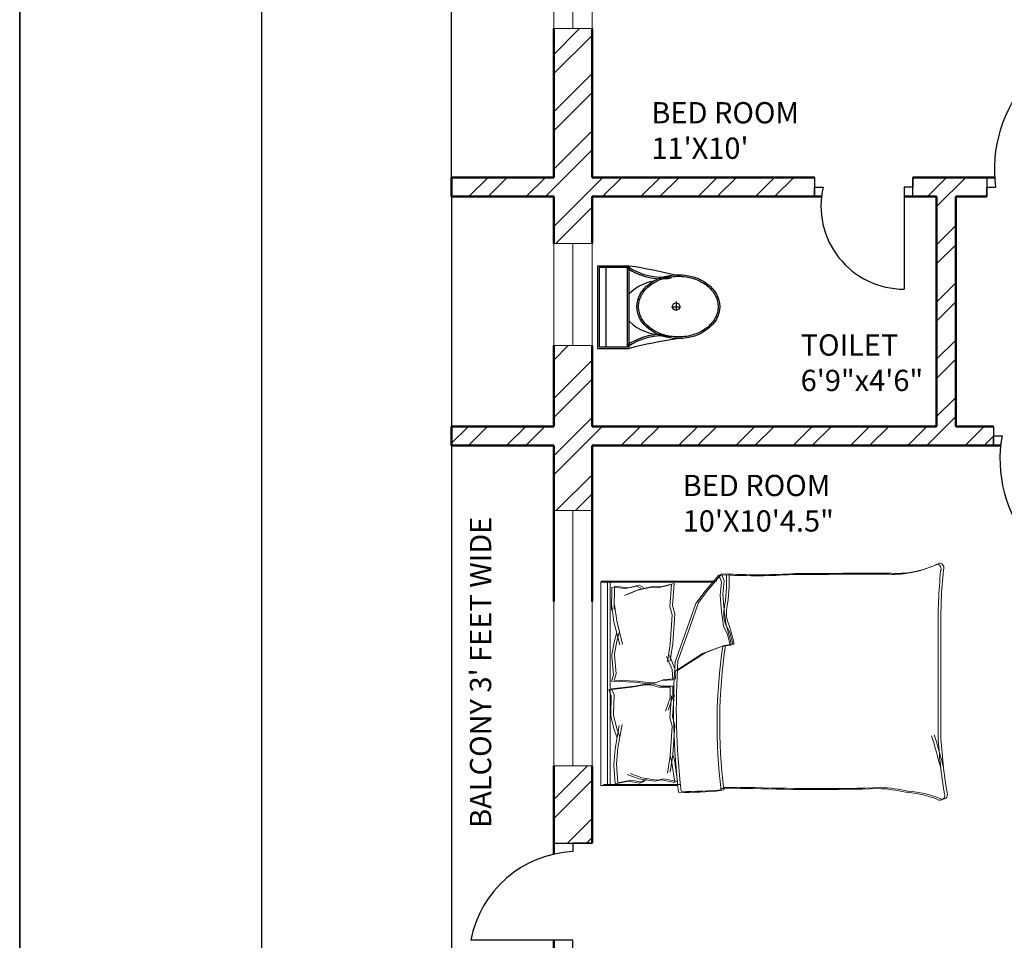
# Model space of a CAD drawing. Units: inches. Extents: x 1980 to 2738, y 1471 to 2568.
# Tile 16 of 22: x 1980 to 2211, y 2112 to 2329. Entities that reach past the tile are written whole.
import ezdxf

# ---------------------------------------------------------------- set-up
doc = ezdxf.new("R2010")
doc.units = ezdxf.units.IN
for name, color, linetype, lineweight in [('A-ANNO-DIMS', 2, 'Continuous', 18), ('A-ANNO-TTLB', 7, 'Continuous', 35), ('A-AREA-IDEN', 7, 'Continuous', 18), ('A-DOOR', 31, 'Continuous', 25), ('A-FLOR-BALC', 7, 'Continuous', 25), ('A-FLOR-FIXT', 8, 'Continuous', 25), ('A-FURN', 8, 'Continuous', 18), ('A-GLAZ', 141, 'Continuous', 18), ('A-WALL', 7, 'Continuous', 50)]:
    doc.layers.add(name, color=color, linetype=linetype, lineweight=lineweight)
doc.layers.add('A-WALL-PATT', color=9, linetype='Continuous', lineweight=13, true_color=0xd19cc7)
doc.styles.get("Standard").update_dxf_attribs({"font": 'arial.ttf'})
doc.dimstyles.get("Standard").update_dxf_attribs({"dimtxt": 0.18, "dimasz": 0.18, "dimexe": 0.18, "dimexo": 0.0625, "dimgap": 0.09, "dimtad": 0, "dimtih": 1, "dimtoh": 1, "dimdec": 4, "dimzin": 0, "dimdsep": 46, "dimtxsty": 'Standard', "dimcen": 0.09, "dimadec": 0, "dimazin": 0, "dimtfac": 1, "dimtdec": 4, "dimtofl": 0, "dimtmove": 0, "dimatfit": 3, "dimfxl": 1, "dimtolj": 1, "dimtzin": 0, "dimarcsym": 0})

# ---------------------------------------------------------------- blocks, each defined once
blk = doc.blocks.new('A$C31115884')
for p, q in [((283.1, 497.7), (223.4, 497.7)), ((257.5, 466.4), (257.5, 523.2)), ((0, 200), (0, 0)), ((520, 200), (0, 200)), ((10, 190), (10, 10)), ((510, 190), (10, 190)), ((510, 10), (510, 190)), ((520, 0), (520, 200)), ((510, 54.5), (0, 54.5)), ((10, 10), (510, 10)), ((0, 0), (520, 0))]:
    blk.add_line(p, q)
blk.add_circle((255.6, 496.4), 23.6)
for centre, radius, start, end in [((2777.7, -204.6), 2807, 165.4549, 171.71327), ((3237, 905), 2807, 188.28673, 194.5451), ((-294.5, 403.3), 364.7, 324.20913, 9.34987), ((-294.5, 403.3), 374.7, 324.20913, 9.34987), ((805.8, 403.3), 364.7, 170.65013, 215.79087), ((139.5, 406.2), 293.5, 315.84364, 2.65635), ((805.8, 403.3), 374.7, 179.20365, 215.79087), ((383.6, 406.2), 293.5, 190.27735, 224.15636)]:
    blk.add_arc(centre, radius, start, end)
blk.add_ellipse((256.2, 509.9), major_axis=(0, -260.7), ratio=0.772727)
blk.add_open_spline([(256.2, 259.2), (263.1, 259.2), (270, 259.7), (287.8, 262.3), (298.7, 265.1), (319.9, 273.1), (330.2, 278.4), (350.1, 291.1), (359.7, 298.7), (377.7, 315.9), (386.2, 325.5), (401.7, 346.6), (408.8, 358.1), (421.3, 382.5), (426.8, 395.5), (435.9, 422.4), (439.5, 436.4), (444.8, 465.1), (446.5, 479.7), (447.9, 509.2), (447.6, 524), (445, 553.3), (442.7, 567.8), (436.3, 596), (432.1, 609.7), (421.9, 636), (416, 648.6), (402.5, 672.1), (395, 683), (378.6, 703), (369.8, 712.1), (351.1, 728), (341.3, 734.8), (320.9, 746.2), (310.4, 750.7), (288.9, 757.3), (278, 759.4), (256, 761), (245, 760.6), (223.1, 757.2), (212.3, 754.3), (191.1, 746.1), (180.8, 740.7), (160.9, 727.8), (151.4, 720.1), (133.5, 702.7), (125.1, 693), (109.6, 671.7), (102.6, 660.2), (90.2, 635.7), (84.9, 622.7), (76, 595.6), (72.4, 581.6), (67.2, 552.9), (65.6, 538.2), (64.4, 508.8), (64.8, 494), (67.5, 464.7), (69.9, 450.2), (76.6, 422), (80.8, 408.3), (91.1, 382.2), (97.2, 369.7), (110.8, 346.3), (118.4, 335.4), (134.8, 315.6), (143.7, 306.7), (162.4, 290.9), (172.3, 284.2), (192.8, 273), (203.3, 268.6), (224.8, 262.2), (235.8, 260.2), (249.9, 259.3), (253, 259.2), (256.2, 259.2)], degree=3, knots=[0, 0, 0, 0, 0.110105, 0.110105, 0.285049, 0.285049, 0.459994, 0.459994, 0.634938, 0.634938, 0.809882, 0.809882, 0.984827, 0.984827, 1.159771, 1.159771, 1.334715, 1.334715, 1.50966, 1.50966, 1.684604, 1.684604, 1.859549, 1.859549, 2.034493, 2.034493, 2.209437, 2.209437, 2.384382, 2.384382, 2.559326, 2.559326, 2.73427, 2.73427, 2.909215, 2.909215, 3.084159, 3.084159, 3.259103, 3.259103, 3.434048, 3.434048, 3.608992, 3.608992, 3.783936, 3.783936, 3.958881, 3.958881, 4.133825, 4.133825, 4.30877, 4.30877, 4.483714, 4.483714, 4.658658, 4.658658, 4.833603, 4.833603, 5.008547, 5.008547, 5.183491, 5.183491, 5.358436, 5.358436, 5.53338, 5.53338, 5.708324, 5.708324, 5.883269, 5.883269, 6.058213, 6.058213, 6.233158, 6.233158, 6.283185, 6.283185, 6.283185, 6.283185])
blk = doc.blocks.new('BED-DOUBLE')
for p, q in [((0, 51.49), (0.64, 51.49)), ((0, 51.27), (26.61, 51.27)), ((0, 51.27), (26.61, 51.27)), ((0, 51.27), (0, 3.48)), ((0.64, 51.49), (27.25, 51.49)), ((0.64, 51.49), (27.25, 51.49)), ((1.53, 3.48), (1.53, 51.27)), ((1.53, 3.48), (1.53, 51.27)), ((2.17, 3.7), (2.17, 51.49)), ((2.17, 3.7), (2.17, 51.49)), ((17.21, 50.93), (14.07, 50.15)), ((17.21, 50.93), (14.07, 50.15)), ((16.81, 45.8), (17.21, 50.93)), ((16.81, 45.79), (17.21, 50.93)), ((27.75, 52.87), (24.5, 49.16)), ((27.75, 52.87), (24.5, 49.16)), ((28.38, 53.1), (25.13, 49.39)), ((28.38, 53.1), (25.13, 49.39)), ((29.49, 52.95), (27.75, 52.87, 3.87)), ((29.49, 52.95), (27.75, 52.87, 3.87)), ((28.36, 51.33), (27.75, 52.87)), ((28.36, 51.33), (27.75, 52.87)), ((28.06, 48.23), (28.36, 51.33)), ((28.06, 48.23), (28.36, 51.33)), ((30.13, 53.18), (28.38, 53.1, 3.87)), ((30.13, 53.18), (28.38, 53.1, 3.87)), ((29, 51.56), (28.38, 53.1)), ((29, 51.56), (28.38, 53.1)), ((28.69, 48.46), (29, 51.56)), ((28.69, 48.46), (29, 51.56)), ((2.56, 50.11), (2.46, 44.71)), ((2.56, 50.11), (2.46, 44.71)), ((2.56, 50.11), (5.77, 49.73)), ((2.56, 50.11), (5.77, 49.73)), ((3.2, 50.34), (3.1, 44.94)), ((3.2, 50.34), (3.1, 44.94)), ((3.2, 50.34), (6.41, 49.96)), ((3.2, 50.34), (6.41, 49.96)), ((8.26, 49.31), (5.58, 48.13)), ((8.26, 49.31), (5.58, 48.13)), ((5.77, 49.73), (8.34, 50.33)), ((5.77, 49.73), (8.34, 50.33)), ((8.9, 49.54), (6.22, 48.36)), ((8.9, 49.54), (6.22, 48.36)), ((6.41, 49.96), (8.98, 50.56)), ((6.41, 49.96), (8.98, 50.56)), ((11.83, 50.11), (8.26, 49.31)), ((11.83, 50.11), (8.26, 49.31)), ((8.34, 50.33), (9.38, 49.81)), ((8.34, 50.33), (9.38, 49.81)), ((12.47, 50.34), (8.9, 49.54)), ((12.47, 50.34), (8.9, 49.54)), ((8.98, 50.56), (10.02, 50.04)), ((8.98, 50.56), (10.02, 50.04)), ((13.43, 49.92), (11.83, 50.11)), ((13.43, 49.92), (11.83, 50.11)), ((14.07, 50.15), (12.47, 50.34)), ((14.07, 50.15), (12.47, 50.34)), ((16.57, 50.7), (13.43, 49.92)), ((16.57, 50.7), (13.43, 49.92)), ((16.17, 45.57), (16.57, 50.7)), ((16.17, 45.57), (16.57, 50.7)), ((24.5, 49.16), (22.33, 46.22)), ((24.5, 49.16), (22.33, 46.22)), ((25.13, 49.39), (22.97, 46.45)), ((25.13, 49.39), (22.97, 46.45)), ((22.97, 46.45), (20.96, 40.87)), ((22.97, 46.45), (20.96, 40.87)), ((28.36, 44.36), (28.06, 48.23)), ((28.36, 44.36), (28.06, 48.23)), ((29, 44.59), (28.69, 48.46)), ((29, 44.59), (28.69, 48.46)), ((2.46, 44.71), (2.54, 45.71)), ((2.46, 44.71), (2.54, 45.71)), ((2.54, 45.71), (3.07, 41.91)), ((2.54, 45.71), (3.07, 41.91)), ((3.1, 44.94), (3.18, 45.94)), ((3.1, 44.94), (3.18, 45.94)), ((3.18, 45.94), (3.71, 42.14)), ((3.18, 45.94), (3.71, 42.14)), ((16.73, 43.61), (16.17, 45.57)), ((16.73, 43.61), (16.17, 45.57)), ((17.37, 43.83), (16.81, 45.8)), ((17.37, 43.83), (16.81, 45.79)), ((22.33, 46.22), (20.32, 40.64)), ((22.33, 46.22), (20.32, 40.64)), ((28.83, 40.95), (28.36, 44.36)), ((28.83, 40.95), (28.36, 44.36)), ((29.47, 41.18), (29, 44.59)), ((29.47, 41.18), (29, 44.59)), ((3.07, 41.91), (4.42, 36.5)), ((3.07, 41.91), (4.42, 36.5)), ((3.71, 42.14), (5.06, 36.72)), ((3.71, 42.14), (5.06, 36.72)), ((16.29, 36.6), (16.73, 43.61)), ((16.29, 36.6), (16.73, 43.61)), ((16.93, 36.82), (17.37, 43.83)), ((16.93, 36.82), (17.37, 43.83)), ((4.31, 39.43), (3.72, 37.36)), ((4.31, 39.43), (3.72, 37.36)), ((20.32, 40.64), (17.38, 32.31)), ((20.32, 40.64), (17.38, 32.31)), ((20.96, 40.87), (18.02, 32.53)), ((20.96, 40.87), (18.02, 32.53)), ((29.76, 38.94), (28.83, 40.95)), ((29.76, 38.94), (28.83, 40.95)), ((30.4, 39.17), (29.47, 41.18)), ((30.4, 39.17), (29.47, 41.18)), ((79.24, 15.06), (79.24, 39.68)), ((79.24, 15.06), (79.24, 39.68)), ((79.88, 15.29), (79.88, 39.91)), ((79.88, 15.29), (79.88, 39.91)), ((3.08, 37.14), (2.54, 34.2)), ((3.08, 37.14), (2.54, 34.2)), ((3.67, 39.2), (3.08, 37.14)), ((3.67, 39.2), (3.08, 37.14)), ((3.72, 37.36), (3.18, 34.43)), ((3.72, 37.36), (3.18, 34.43)), ((30.38, 36.46), (29.76, 38.94)), ((30.38, 36.46), (29.76, 38.94)), ((31.02, 36.69), (30.4, 39.17)), ((31.02, 36.69), (30.4, 39.17)), ((15.63, 32.56), (16.29, 36.6)), ((15.63, 32.56), (16.29, 36.6)), ((16.27, 32.79), (16.93, 36.82)), ((16.27, 32.79), (16.93, 36.82)), ((23.88, 34.45), (28.36, 36.15)), ((23.88, 34.45), (28.36, 36.15)), ((24.52, 34.68), (29, 36.38)), ((24.52, 34.68), (29, 36.38)), ((28.36, 36.15), (30.38, 36.46)), ((28.36, 36.15), (30.38, 36.46)), ((29, 36.38), (31.02, 36.69)), ((29, 36.38), (31.02, 36.69)), ((2.54, 34.2), (2.56, 33.88)), ((2.54, 34.2), (2.56, 33.88)), ((2.56, 33.88), (2.98, 29.46)), ((2.56, 33.88), (2.98, 29.46)), ((3.18, 34.43), (3.2, 34.11)), ((3.18, 34.43), (3.2, 34.11)), ((3.2, 34.11), (3.62, 29.68)), ((3.2, 34.11), (3.62, 29.68)), ((16.74, 30.75), (15.45, 33.82)), ((16.74, 30.75), (15.45, 33.82)), ((17.38, 30.98), (16.09, 34.05)), ((17.38, 30.98), (16.09, 34.05)), ((17.38, 30.26), (23.88, 34.45)), ((17.38, 30.26), (23.88, 34.45)), ((18.02, 30.49), (24.52, 34.68)), ((18.02, 30.49), (24.52, 34.68)), ((16.89, 28.3), (16.74, 30.75)), ((16.89, 28.3), (16.74, 30.75)), ((17.53, 28.53), (17.38, 30.98)), ((17.53, 28.53), (17.38, 30.98)), ((2.98, 29.46), (2.49, 27.98)), ((2.98, 29.46), (2.49, 27.98)), ((2.49, 27.98), (7.87, 27.73)), ((2.49, 27.98), (7.87, 27.73)), ((3.62, 29.68), (3.13, 28.21)), ((3.62, 29.68), (3.13, 28.21)), ((3.13, 28.21), (8.51, 27.96)), ((3.13, 28.21), (8.51, 27.96)), ((8.51, 27.96), (11.72, 27.58)), ((8.51, 27.96), (11.72, 27.58)), ((12.38, 27.44), (14.22, 28.13)), ((12.38, 27.44), (14.22, 28.13)), ((13.02, 27.66), (14.86, 28.36)), ((13.02, 27.66), (14.86, 28.36)), ((14.22, 28.13), (16.89, 28.3)), ((14.22, 28.13), (16.89, 28.3)), ((14.86, 28.36), (17.53, 28.53)), ((14.86, 28.36), (17.53, 28.53)), ((1.87, 25.98), (7.22, 26.56)), ((1.87, 25.98), (7.22, 26.56)), ((2.45, 24.54), (1.87, 25.98)), ((2.45, 24.54), (1.87, 25.98)), ((2.51, 26.21), (7.86, 26.79)), ((2.51, 26.21), (7.86, 26.79)), ((3.09, 24.77), (2.51, 26.21)), ((3.09, 24.77), (2.51, 26.21)), ((7.22, 26.56), (10.4, 27.14)), ((7.22, 26.56), (10.4, 27.14)), ((7.86, 26.79), (11.04, 27.37)), ((7.86, 26.79), (11.04, 27.37)), ((7.87, 27.73), (11.08, 27.36)), ((7.87, 27.73), (11.08, 27.35)), ((10.4, 27.14), (11.7, 27.14)), ((10.4, 27.14), (11.7, 27.14)), ((11.04, 27.37), (12.34, 27.37)), ((11.04, 27.37), (12.34, 27.37)), ((11.08, 27.36), (12.38, 27.44)), ((11.08, 27.35), (12.38, 27.44)), ((11.7, 27.14), (13.58, 26.56)), ((11.7, 27.14), (13.58, 26.56)), ((11.72, 27.58), (13.02, 27.66)), ((11.72, 27.58), (13.02, 27.66)), ((12.34, 27.37), (14.22, 26.79)), ((12.34, 27.37), (14.22, 26.79)), ((13.58, 26.56), (16.26, 26.56)), ((13.58, 26.56), (16.26, 26.56)), ((14.22, 26.79), (16.9, 26.79)), ((14.22, 26.79), (16.9, 26.79)), ((16.26, 26.56), (16.26, 24.1)), ((16.26, 26.56), (16.26, 24.1)), ((16.9, 26.79), (16.9, 24.33)), ((16.9, 26.79), (16.9, 24.33)), ((2.3, 20.09), (2.45, 24.54)), ((2.3, 20.09), (2.45, 24.54)), ((2.94, 20.32), (3.09, 24.77)), ((2.94, 20.32), (3.09, 24.77)), ((16.26, 24.1), (15.17, 20.96)), ((16.26, 24.1), (15.17, 20.96)), ((16.9, 24.33), (15.81, 21.19)), ((16.9, 24.33), (15.81, 21.19)), ((16.17, 19.38), (16.57, 24.52)), ((16.17, 19.38), (16.57, 24.52)), ((16.81, 19.61), (17.21, 24.74)), ((16.81, 19.61), (17.21, 24.74)), ((2.3, 19.77), (2.3, 20.09)), ((2.3, 19.77), (2.3, 20.09)), ((3.03, 16.88), (2.3, 19.77)), ((3.03, 16.88), (2.3, 19.77)), ((2.94, 20), (2.94, 20.32)), ((2.94, 20), (2.94, 20.32)), ((3.67, 17.11), (2.94, 20)), ((3.67, 17.11), (2.94, 20)), ((16.73, 17.42), (16.17, 19.38)), ((16.73, 17.42), (16.17, 19.38)), ((17.37, 17.65), (16.81, 19.61)), ((17.37, 17.65), (16.81, 19.61)), ((3.75, 14.86), (3.03, 16.88)), ((3.75, 14.85), (3.03, 16.88)), ((3.32, 12.11), (4.33, 17.6)), ((3.32, 12.11), (4.33, 17.6)), ((4.39, 15.08), (3.67, 17.11)), ((4.39, 15.08), (3.67, 17.11)), ((3.96, 12.34), (4.97, 17.83)), ((3.96, 12.34), (4.97, 17.83)), ((16.29, 10.41), (16.73, 17.42)), ((16.29, 10.41), (16.73, 17.42)), ((16.93, 10.64), (17.37, 17.65)), ((16.93, 10.64), (17.37, 17.65)), ((3.03, 8.29), (3.32, 12.11)), ((3.03, 8.28), (3.32, 12.11)), ((3.67, 8.51), (3.96, 12.34)), ((3.67, 8.51), (3.96, 12.34)), ((15.63, 6.38), (16.29, 10.41)), ((15.63, 6.38), (16.29, 10.41)), ((16.27, 6.61), (16.93, 10.64)), ((16.27, 6.61), (16.93, 10.64)), ((16.29, 10.41), (16.62, 9.28)), ((16.29, 10.41), (16.62, 9.28)), ((16.62, 9.28), (17.34, 4.18)), ((16.62, 9.28), (17.34, 4.18)), ((16.93, 10.64), (17.26, 9.51)), ((16.93, 10.64), (17.26, 9.51)), ((17.26, 9.51), (17.98, 4.41)), ((17.26, 9.51), (17.98, 4.41)), ((3.01, 8.18), (3.03, 8.29)), ((3.01, 8.18), (3.03, 8.28)), ((3.34, 3.9), (3.01, 8.18)), ((3.34, 3.9), (3.01, 8.18)), ((3.65, 8.41), (3.67, 8.51)), ((3.65, 8.41), (3.67, 8.51)), ((3.98, 4.13), (3.65, 8.41)), ((3.98, 4.13), (3.65, 8.41)), ((3.96, 4.12), (7.14, 4.7)), ((3.96, 4.12), (7.14, 4.7)), ((8.95, 5.05), (6.21, 6.06)), ((8.95, 5.05), (6.21, 6.06)), ((9.59, 5.28), (6.85, 6.29)), ((9.59, 5.28), (6.85, 6.29)), ((7.14, 4.7), (9.74, 4.27)), ((7.14, 4.7), (9.74, 4.27)), ((12.57, 4.47), (8.95, 5.05)), ((12.57, 4.47), (8.95, 5.05)), ((13.21, 4.7), (9.59, 5.28)), ((13.21, 4.7), (9.59, 5.28)), ((9.74, 4.27), (10.75, 4.85)), ((9.74, 4.27), (10.75, 4.85)), ((14.16, 4.76), (12.57, 4.47)), ((14.16, 4.76), (12.57, 4.47)), ((14.8, 4.99), (13.21, 4.7)), ((14.8, 4.99), (13.21, 4.7)), ((17.34, 4.18), (14.16, 4.76)), ((17.34, 4.18), (14.16, 4.76)), ((17.98, 4.41), (14.8, 4.99)), ((17.98, 4.41), (14.8, 4.99)), ((18.11, 3.48), (0, 3.48)), ((18.11, 3.48), (0, 3.48)), ((18.75, 3.7), (0.64, 3.7)), ((18.75, 3.7), (0.64, 3.7)), ((3.32, 3.89), (6.5, 4.47)), ((3.32, 3.89), (6.5, 4.47)), ((6.5, 4.47), (9.1, 4.04)), ((6.5, 4.47), (9.1, 4.04)), ((9.1, 4.04), (10.11, 4.62)), ((9.1, 4.04), (10.11, 4.62))]:
    blk.add_line(p, q)
for centre, radius, start, end in [((69.31, 76.39), 23.07, 267.4714, 296.4681), ((69.31, 76.39), 23.07, 267.4714, 296.4681), ((79.51, 54.64), 1.1, 332.6588, 86.02), ((79.51, 54.64), 1.1, 332.6588, 86.02), ((36.95, 182.49), 129.5, 266.9791, 273.8365), ((36.95, 182.49), 129.5, 266.9791, 273.8365), ((68.46, -4508.51), 4561.86, 90.00217, 90.28689), ((68.46, -4508.52), 4561.86, 90.00217, 90.28689), ((68.67, 76.16), 23.07, 267.4714, 296.4681), ((68.67, 76.16), 23.07, 267.4714, 296.4681), ((78.87, 54.41), 1.1, 332.6588, 86.02), ((78.87, 54.41), 1.1, 332.6588, 86.02), ((212.28, 41.15), 133.04, 174.4998, 180.6351), ((212.28, 41.15), 133.04, 174.4998, 180.6351), ((212.92, 41.38), 133.04, 174.4998, 180.6351), ((212.92, 41.38), 133.04, 174.4998, 180.6351), ((-6.66, 51.33), 36.18, 349.8763, 2.5657), ((-6.66, 51.33), 36.18, 349.8763, 2.5657), ((36.31, 182.27), 129.5, 266.9791, 273.8365), ((36.31, 182.27), 129.5, 266.9791, 273.8365), ((-6.02, 51.56), 36.18, 349.8763, 2.5657), ((-6.02, 51.56), 36.18, 349.8763, 2.5657), ((67.82, -4508.74), 4561.86, 90.00217, 90.28689), ((67.82, -4508.74), 4561.86, 90.00217, 90.28689), ((35.07, 43.74), 6.22, 168.6608, 203.7384), ((35.07, 43.74), 6.22, 168.6608, 203.7384), ((35.71, 43.97), 6.22, 168.6608, 203.7384), ((35.71, 43.97), 6.22, 168.6608, 203.7384), ((1.48, 31.15), 29.65, 10.6617, 19.8806), ((1.48, 31.15), 29.65, 10.6617, 19.8806), ((2.12, 31.38), 29.65, 10.6617, 19.8806), ((2.12, 31.38), 29.65, 10.6617, 19.8806), ((156.32, 17.76), 129.02, 171.7845, 186.9006), ((156.32, 17.76), 129.02, 171.7845, 186.9006), ((156.96, 17.98), 129.02, 171.7845, 186.9006), ((156.96, 17.98), 129.02, 171.7845, 186.9006), ((30.44, 36.64), 0.185, 250.2464, 1.1377), ((30.44, 36.64), 0.185, 250.2464, 1.1377), ((31.08, 36.86), 0.185, 250.2464, 1.1377), ((31.08, 36.86), 0.185, 250.2464, 1.1377), ((182.05, 21.36), 164.97, 176.0865, 186.7821), ((182.05, 21.36), 164.97, 176.0865, 186.7821), ((182.69, 21.59), 164.97, 176.0865, 186.7821), ((182.69, 21.59), 164.97, 176.0865, 186.7821), ((-23.71, -17.22), 106.46, 13.3832, 17.7053), ((-23.71, -17.22), 106.46, 13.3832, 17.7053), ((-23.07, -16.99), 106.46, 13.3832, 17.7053), ((-23.07, -16.99), 106.46, 13.3832, 17.7053), ((200.84, 21.43), 121.76, 182.9958, 189.4091), ((200.84, 21.43), 121.76, 182.9958, 189.4091), ((201.48, 21.66), 121.76, 182.9958, 189.4091), ((201.48, 21.66), 121.76, 182.9958, 189.4091), ((20.74, 85.39), 83.31, 268.7218, 275.604), ((20.74, 85.39), 83.31, 268.7218, 275.604), ((31.17, -167.31), 170.11, 88.4762, 91.0082), ((31.17, -167.31), 170.11, 88.4762, 91.0082), ((31.81, -167.08), 170.11, 88.4762, 91.0082), ((31.81, -167.08), 170.11, 88.4762, 91.0082), ((50.61, 484.82), 482.31, 268.2277, 271.7185), ((50.61, 484.82), 482.31, 268.2277, 271.7185), ((51.25, 485.05), 482.31, 268.2277, 271.7185), ((51.25, 485.05), 482.31, 268.2277, 271.7185), ((64.51, -26.9), 29.63, 76.0648, 88.9113), ((64.51, -26.9), 29.63, 76.0648, 88.9113), ((65.15, -26.67), 29.63, 76.0648, 88.9113), ((65.15, -26.67), 29.63, 76.0648, 88.9113), ((20.1, 85.16), 83.31, 268.7218, 275.604), ((20.1, 85.16), 83.31, 268.7218, 275.604), ((70.28, -21.66), 23.56, 67.9751, 86.652), ((70.28, -21.66), 23.56, 67.9751, 86.652), ((70.91, -21.43), 23.56, 67.9751, 86.652), ((70.91, -21.43), 23.56, 67.9751, 86.652), ((79.72, 1.09), 1.09, 236.1736, 23.4781), ((79.72, 1.09), 1.09, 236.1736, 23.4781), ((80.36, 1.32), 1.09, 236.1736, 23.4781), ((80.36, 1.32), 1.09, 236.1736, 23.4781)]:
    blk.add_arc(centre, radius, start, end)
blk = doc.blocks.new('WIN-60IN-WALL')
for p, q in [((0, 9), (0, 0)), ((60, 9), (0, 9)), ((60, 4.5), (60, 9)), ((60, 9), (60, 0)), ((0, 0), (0, 4.5)), ((0, 4.5), (60, 4.5)), ((0, 0), (60, 0))]:
    blk.add_line(p, q)
blk = doc.blocks.new('WIN-24IN-WALL')
for p, q in [((4.5, 24), (0, 24)), ((0, 24), (9, 24)), ((0, 24), (0, 0)), ((4.5, 0), (4.5, 24)), ((9, 0), (9, 24)), ((0, 0), (9, 0)), ((9, 0), (4.5, 0))]:
    blk.add_line(p, q)
blk = doc.blocks.new('*D35')
at = {"layer": 'A-ANNO-DIMS', "color": 0, "lineweight": -2, "transparency": 16777216}
for p, q in [((2081.08, 2291.77), (2081.08, 2507.54)), ((2081.26, 2507.36), (2362.79, 2507.36)), ((2644.9, 2507.36), (2363.37, 2507.36)), ((2645.08, 2291.77), (2645.08, 2507.54))]:
    blk.add_line(p, q, dxfattribs=at)
at = {"layer": 'A-ANNO-DIMS', "color": 0, "transparency": 16777216}
for points in [[(2081.26, 2507.39), (2081.26, 2507.33), (2081.08, 2507.36)], [(2644.9, 2507.39), (2644.9, 2507.33), (2645.08, 2507.36)]]:
    blk.add_solid(points, dxfattribs=at)
at = {"layer": 'Defpoints', "color": 0, "transparency": 16777216}
for p in [(2645.08, 2507.36), (2081.08, 2291.71), (2645.08, 2291.71)]:
    blk.add_point(p, dxfattribs=at)
at = {"layer": 'A-ANNO-DIMS', "color": 0, "transparency": 16777216, "insert": (2363.08, 2507.36), "char_height": 0.18, "attachment_point": 5}
blk.add_mtext('\\A1;564', dxfattribs=at)
blk = doc.blocks.new('*D36')
at = {"layer": 'A-ANNO-DIMS', "color": 0, "lineweight": -2, "transparency": 16777216}
for p, q in [((2105.02, 2462.71), (2036.25, 2462.71)), ((2036.43, 2462.53), (2036.43, 2053.39)), ((2036.43, 1643.89), (2036.43, 2053.02)), ((2105.02, 1643.71), (2036.25, 1643.71))]:
    blk.add_line(p, q, dxfattribs=at)
at = {"layer": 'A-ANNO-DIMS', "color": 0, "transparency": 16777216}
for points in [[(2036.4, 2462.53), (2036.46, 2462.53), (2036.43, 2462.71)], [(2036.4, 1643.89), (2036.46, 1643.89), (2036.43, 1643.71)]]:
    blk.add_solid(points, dxfattribs=at)
at = {"layer": 'Defpoints', "color": 0, "transparency": 16777216}
for p in [(2036.43, 2462.71), (2105.08, 2462.71), (2105.08, 1643.71)]:
    blk.add_point(p, dxfattribs=at)
at = {"layer": 'A-ANNO-DIMS', "color": 0, "transparency": 16777216, "insert": (2036.43, 2053.21), "char_height": 0.18, "attachment_point": 5}
blk.add_mtext('\\A1;819', dxfattribs=at)

msp = doc.modelspace()

# ---------------------------------------------------------------- hatches: boundary and pattern name
at = {"layer": 'A-WALL-PATT'}
h = msp.add_hatch(dxfattribs=at)
h.set_pattern_fill('ANSI32', color=256)
h.paths.add_polyline_path([(2257.5661, 2416.2064), (2257.5661, 2420.7064), (2250.5833, 2420.7064), (2250.5833, 2462.7064), (2246.0833, 2462.7064), (2246.0833, 2420.7064), (2237.0791, 2420.7064), (2237.0791, 2411.7064), (2246.0833, 2411.7064), (2246.0833, 2291.7064), (2242.6109, 2291.7064), (2242.6109, 2287.2064), (2246.0833, 2287.2064), (2250.5833, 2287.2064), (2250.5833, 2291.7064), (2250.5833, 2411.7064), (2257.5661, 2411.7064)])
h.paths.add_polyline_path([(2387.0396, 2416.2064), (2387.0396, 2420.7064), (2367.5833, 2420.7064), (2367.5833, 2462.7064), (2358.5833, 2462.7064), (2358.5833, 2420.7064), (2329.3087, 2420.7064), (2329.3087, 2411.7064), (2358.5833, 2411.7064), (2358.5833, 2321.7275), (2358.5833, 2309.7064), (2347.3089, 2309.7064), (2293.3089, 2309.7064), (2293.3089, 2259.0771), (2297.8089, 2259.0771), (2297.8089, 2305.2064), (2347.3089, 2305.2064), (2347.3089, 2284.7412), (2351.8089, 2284.7412), (2351.8089, 2305.2064), (2372.3188, 2305.2064), (2372.3761, 2284.3899), (2377.0295, 2284.3899), (2377.0295, 2299.3058), (2377.0295, 2305.2064), (2426.5295, 2305.2064), (2426.5295, 2257.5573), (2431.0295, 2257.5573), (2431.0295, 2309.7064), (2377.0295, 2309.7064), (2367.5833, 2309.7064), (2367.5833, 2321.7275), (2367.5833, 2411.7064), (2387.0396, 2411.7064)])
h.paths.add_polyline_path([(2448.5267, 2416.2064), (2448.5267, 2420.7064), (2423.0396, 2420.7064), (2423.0396, 2411.7064), (2448.5267, 2411.7064)])
h.paths.add_polyline_path([(2130.9128, 2416.2064), (2130.9128, 2420.7064), (2105.0833, 2420.7064), (2105.0833, 2386.6942), (2114.0833, 2386.6942), (2114.0833, 2411.7064), (2130.9128, 2411.7064)])
h.paths.add_polyline_path([(2212.9478, 2420.7064), (2190.9128, 2420.7064), (2190.9128, 2411.7064), (2212.9478, 2411.7064), (2212.9478, 2416.2064)])
h.paths.add_polyline_path([(2114.0833, 2326.6942), (2105.0833, 2326.6942), (2105.0833, 2291.7064), (2081.0833, 2291.7064), (2081.0833, 2287.2064), (2105.0833, 2287.2064), (2105.0833, 2276.1935), (2114.0833, 2276.1935), (2114.0833, 2287.2064), (2166.3825, 2287.2064), (2166.3825, 2289.4564), (2166.3825, 2291.7064), (2114.0833, 2291.7064)])
h.paths.add_polyline_path([(2114.0833, 2252.1935), (2105.0833, 2252.1935), (2105.0833, 2233.2064), (2081.0833, 2233.2064), (2081.0833, 2228.7064), (2105.0833, 2228.7064), (2105.0833, 2213.4478), (2114.0833, 2213.4478), (2114.0833, 2228.7064), (2195.0833, 2228.7064), (2199.5833, 2228.7064), (2208.4455, 2228.7064), (2208.4455, 2230.9564), (2208.4455, 2233.2064), (2199.5833, 2233.2064), (2199.5833, 2287.2064), (2206.8904, 2287.2064), (2206.8904, 2289.4564), (2206.8904, 2291.7064), (2189.446, 2291.7064), (2189.446, 2289.4564), (2189.446, 2287.2064), (2195.0833, 2287.2064), (2195.0833, 2233.2064), (2114.0833, 2233.2064)])
h.paths.add_polyline_path([(2114.0833, 2153.4478), (2109.5833, 2153.4478), (2105.0833, 2153.4478), (2105.0833, 2135.2374), (2114.0833, 2135.2374)], flags=17)
h.paths.add_polyline_path([(2135.9619, 2095.4081), (2140.1805, 2095.4081), (2140.1805, 2104.2064), (2114.0833, 2104.2064), (2114.0833, 2110.3997), (2109.5833, 2110.3997), (2105.0833, 2110.3997), (2105.0833, 2104.2064), (2081.0833, 2104.2064), (2081.0833, 2099.7064), (2105.0833, 2099.7064), (2127.5416, 2099.8532), (2127.5416, 2056.9393), (2136.2133, 2056.9393)], flags=17)
h.paths.add_polyline_path([(2255.4895, 2104.2064), (2250.5833, 2104.2064), (2250.5833, 2233.2064), (2246.0833, 2233.2064), (2242.4941, 2233.2064), (2242.4941, 2228.7064), (2246.0833, 2228.7064), (2246.0833, 2104.2064), (2163.6825, 2104.2064), (2163.6825, 2099.8072), (2163.6825, 2095.4081), (2191.4325, 2095.4081), (2191.4325, 2011.2064), (2186.0833, 2011.2064), (2136.5143, 2010.8824), (2136.3702, 2032.9403), (2131.9559, 2032.9115), (2127.5416, 2032.8826), (2127.5416, 2006.7064), (2105.0833, 2006.7064), (2081.0833, 2006.7064), (2081.0833, 2002.2064), (2105.0833, 2002.2064), (2105.0833, 1995.9329), (2114.0833, 1995.9329), (2114.0833, 2002.2064), (2246.0833, 2002.2064), (2246.0833, 1877.7064), (2242.1358, 1877.7064), (2242.1358, 1873.2064), (2250.5833, 1873.2064), (2250.5833, 2002.2064), (2255.3335, 2002.2064), (2255.3335, 2011.2064), (2195.9325, 2011.2064), (2195.9325, 2095.2064), (2255.4895, 2095.2064), (2255.4895, 2099.5471)])
h.paths.add_polyline_path([(2199.5833, 1873.2064), (2209.827, 1873.2064), (2209.827, 1875.4564), (2209.827, 1877.7064), (2114.0833, 1877.7064), (2114.0833, 1890.0968), (2105.0833, 1890.0968), (2105.0833, 1877.7064), (2081.0833, 1877.7064), (2081.0833, 1873.2064), (2105.0833, 1873.2064), (2105.0833, 1857.7279), (2114.0833, 1857.7279), (2114.0833, 1873.2064), (2195.0833, 1873.2064), (2195.0833, 1819.2064), (2190.298, 1819.2064), (2190.298, 1814.7064), (2209.8976, 1814.7064), (2209.8976, 1816.9564), (2209.8976, 1819.2064), (2199.5833, 1819.2064)])
h.paths.add_polyline_path([(2114.0833, 1814.7064), (2166.2538, 1814.7064), (2166.2538, 1816.9564), (2166.2538, 1819.2064), (2114.0833, 1819.2064), (2114.0833, 1833.7279), (2109.5833, 1833.7279), (2105.0833, 1833.7279), (2105.0833, 1819.2064), (2081.0833, 1819.2064), (2081.0833, 1814.7064), (2105.0833, 1814.7064), (2105.0833, 1782.5516), (2114.0833, 1782.5516)])
h.paths.add_polyline_path([(2114.0833, 1722.5516), (2109.5833, 1722.5516), (2105.0833, 1722.5516), (2105.0833, 1685.7064), (2124.5104, 1685.7064), (2124.5104, 1690.2064), (2124.5104, 1694.7064), (2114.0833, 1694.7064)])
h.paths.add_polyline_path([(2218.8787, 1694.7064), (2184.5104, 1694.7064), (2184.5104, 1685.7064), (2218.8787, 1685.7064), (2218.8787, 1690.2064)])
h.paths.add_polyline_path([(2250.5833, 1819.2064), (2242.6431, 1819.2064), (2242.6431, 1816.9564), (2242.6431, 1814.7064), (2246.0833, 1814.7064), (2246.0833, 1694.7064), (2240.4035, 1694.7064), (2240.4035, 1690.2064), (2240.4035, 1685.7064), (2246.0833, 1685.7064), (2246.0833, 1643.7064), (2250.5833, 1643.7064), (2250.5833, 1685.7064), (2255.9859, 1685.7064), (2255.9859, 1690.2064), (2255.9859, 1694.7064), (2250.5833, 1694.7064)])
h.paths.add_polyline_path([(2297.4764, 1694.7064), (2279.3934, 1694.7064), (2279.3934, 1690.2064), (2279.3934, 1685.7064), (2297.4764, 1685.7064), (2297.4764, 1690.2064)])
h.paths.add_polyline_path([(2377.1596, 1694.7064), (2367.5833, 1694.7064), (2367.5833, 1787.7064), (2431.0295, 1787.7064), (2431.0295, 1792.2064), (2431.0295, 1849.4149), (2428.7795, 1849.4149), (2426.5295, 1849.4149), (2426.5295, 1792.2064), (2421.5833, 1792.2064), (2367.5833, 1792.2064), (2297.8089, 1792.2064), (2297.8089, 1850.2946), (2295.5589, 1850.2946), (2293.3089, 1850.2946), (2293.3089, 1792.2064), (2293.3089, 1787.7064), (2297.8089, 1787.7064), (2358.5833, 1787.7064), (2358.5833, 1694.7064), (2333.4764, 1694.7064), (2333.4764, 1685.7064), (2358.5833, 1685.7064), (2358.5833, 1643.7064), (2367.5833, 1643.7064), (2367.5833, 1685.7064), (2377.1596, 1685.7064)])
h.paths.add_polyline_path([(2442.4912, 1694.7064), (2413.1596, 1694.7064), (2413.1596, 1685.7064), (2442.4912, 1685.7064)])
h.paths.add_polyline_path([(2480.0833, 1814.7064), (2483.4816, 1814.7064), (2483.4816, 1817.9384), (2483.4816, 1819.2064), (2475.5833, 1819.2064), (2475.5833, 1694.7064), (2470.7283, 1694.7064), (2470.7283, 1685.7064), (2475.5833, 1685.7064), (2475.5833, 1643.7064), (2480.0833, 1643.7064), (2480.0833, 1685.7064), (2486.3293, 1685.7064), (2486.3293, 1690.2064), (2486.3293, 1694.7064), (2480.0833, 1694.7064)])
h.paths.add_polyline_path([(2621.0833, 1721.7349), (2612.0833, 1721.7349), (2612.0833, 1694.7064), (2586.1453, 1694.7064), (2586.1453, 1685.7064), (2621.0833, 1685.7064)])
h.paths.add_polyline_path([(2526.1453, 1690.2064), (2526.1453, 1694.7064), (2511.584, 1694.7064), (2511.584, 1690.2064), (2511.584, 1685.7064), (2526.1453, 1685.7064)])
h.paths.add_polyline_path([(2645.0833, 1819.2064), (2621.0833, 1819.2064), (2621.0833, 1835.8527), (2616.5833, 1835.8527), (2612.0833, 1835.8527), (2612.0833, 1819.2064), (2560.2541, 1819.2064), (2560.2541, 1814.7064), (2612.0833, 1814.7064), (2612.0833, 1781.7349), (2621.0833, 1781.7349), (2621.0833, 1814.7064), (2645.0833, 1814.7064)])
h.paths.add_polyline_path([(2645.0833, 1877.7064), (2621.0833, 1877.7064), (2621.0833, 1886.4375), (2612.0833, 1886.4375), (2612.0833, 1877.7064), (2517.1032, 1877.7064), (2517.1032, 1875.4564), (2517.1032, 1873.2064), (2526.5833, 1873.2064), (2526.5833, 1819.2064), (2516.6454, 1819.2064), (2516.6454, 1816.9564), (2516.6454, 1814.7064), (2536.4445, 1814.7064), (2536.4445, 1816.9564), (2536.4445, 1819.2064), (2531.0833, 1819.2064), (2531.0833, 1873.2064), (2612.0833, 1873.2064), (2612.0833, 1859.8527), (2621.0833, 1859.8527), (2621.0833, 1873.2064), (2645.0833, 1873.2064)])
h.paths.add_polyline_path([(2645.0833, 2006.7064), (2621.0833, 2006.7064), (2588.5085, 2006.7064), (2588.5085, 2052.9125), (2579.9045, 2052.9125), (2579.9045, 2011.2064), (2519.9045, 2011.2064), (2519.9045, 2095.2064), (2553.1204, 2095.2064), (2553.1204, 2104.2064), (2480.0833, 2104.2064), (2480.0833, 2228.7064), (2484.3832, 2228.7064), (2484.3832, 2230.9564), (2484.3832, 2233.2064), (2475.5833, 2233.2064), (2475.5833, 2104.2064), (2463.1308, 2104.2064), (2463.1308, 2095.2064), (2501.2463, 2095.2064), (2510.9045, 2095.2064), (2515.4045, 2095.2064), (2515.4045, 2011.2064), (2510.9045, 2011.2064), (2501.2463, 2011.2064), (2462.5957, 2011.2064), (2462.5957, 2002.2064), (2475.5833, 2002.2064), (2475.5833, 1873.2064), (2483.6146, 1873.2064), (2483.6146, 1875.4564), (2483.6146, 1877.7064), (2480.0833, 1877.7064), (2480.0833, 2002.2064), (2612.0833, 2002.2064), (2612.0833, 1996.309), (2621.0833, 1996.309), (2621.0833, 2002.2064), (2645.0833, 2002.2064)])
h.paths.add_polyline_path([(2588.5085, 2099.7277), (2621.0833, 2099.7277), (2645.0833, 2099.7064), (2645.0833, 2104.2064), (2621.0833, 2104.2064), (2621.0833, 2109.0038), (2616.5833, 2109.0038), (2612.0833, 2109.0038), (2612.0833, 2104.2064), (2575.0621, 2104.2064), (2575.0621, 2099.7064), (2575.0621, 2095.2064), (2579.9045, 2095.2064), (2579.9045, 2076.9125), (2588.5085, 2076.9125)], flags=17)
h.paths.add_polyline_path([(2367.5833, 2002.2064), (2373.7228, 2002.2064), (2373.7228, 2006.7064), (2373.7228, 2011.2064), (2350.7889, 2011.2064), (2350.7889, 2006.7064), (2350.7889, 2002.2064), (2358.5833, 2002.2064), (2358.5833, 1877.7064), (2293.3089, 1877.7064), (2293.3089, 1870.4987), (2297.8089, 1870.4987), (2297.8089, 1873.2064), (2347.3089, 1873.2064), (2347.3089, 1847.2208), (2351.8089, 1847.2208), (2351.8089, 1873.2064), (2372.5295, 1873.2064), (2372.5295, 1847.8619), (2377.0295, 1847.8619), (2377.0295, 1873.2064), (2426.5295, 1873.2064), (2426.5295, 1868.7339), (2431.0295, 1868.7339), (2431.0295, 1877.7064), (2367.5833, 1877.7064)])
h.paths.add_polyline_path([(2531.0833, 2287.2064), (2534.2285, 2287.2064), (2534.2285, 2291.7064), (2516.7886, 2291.7064), (2516.7886, 2287.2064), (2526.5833, 2287.2064), (2526.5833, 2233.2064), (2517.9112, 2233.2064), (2517.9112, 2230.9564), (2517.9112, 2228.7064), (2526.5833, 2228.7064), (2531.0833, 2228.7064), (2612.0833, 2228.7064), (2612.0833, 2206.8504), (2621.0833, 2206.8504), (2621.0833, 2228.7064), (2645.0833, 2228.7064), (2645.0833, 2233.2064), (2621.0833, 2233.2064), (2621.0833, 2241.8536), (2616.5833, 2241.8536), (2612.0833, 2241.8536), (2612.0833, 2233.2064), (2531.0833, 2233.2064)])
h.paths.add_polyline_path([(2645.0833, 2291.7064), (2621.0833, 2291.7064), (2621.0833, 2323.0138), (2616.5833, 2323.0138), (2612.0833, 2323.0138), (2612.0833, 2291.7064), (2559.6852, 2291.7064), (2559.6852, 2289.4564), (2559.6852, 2287.2064), (2612.0833, 2287.2064), (2612.0833, 2265.8536), (2621.0833, 2265.8536), (2621.0833, 2287.2064), (2645.0833, 2287.2064)])
h.paths.add_polyline_path([(2621.0833, 2420.7064), (2582.8189, 2420.7064), (2582.8189, 2411.7064), (2612.0833, 2411.7064), (2612.0833, 2383.0138), (2621.0833, 2383.0138)])
h.paths.add_polyline_path([(2480.0833, 2411.7064), (2485.7342, 2411.7064), (2485.7342, 2416.2064), (2485.7342, 2420.7064), (2480.0833, 2420.7064), (2480.0833, 2462.7064), (2475.5833, 2462.7064), (2475.5833, 2420.7064), (2469.4083, 2420.7064), (2469.4083, 2411.7064), (2475.5833, 2411.7064), (2475.5833, 2291.7064), (2475.5833, 2287.2064), (2482.9195, 2287.2064), (2482.9195, 2289.4564), (2482.9195, 2291.7064), (2480.0833, 2291.7064)])
h.paths.add_polyline_path([(2367.5833, 2228.7064), (2431.0295, 2228.7064), (2431.0295, 2233.2064), (2431.0295, 2237.4203), (2428.7795, 2237.4203), (2426.5295, 2237.4203), (2426.5295, 2233.2064), (2377.0295, 2233.2064), (2377.0295, 2260.3837), (2372.4423, 2260.3837), (2372.517, 2233.2635), (2351.8089, 2233.2064), (2351.8089, 2260.7412), (2347.3089, 2260.7412), (2347.3089, 2233.2064), (2297.8089, 2233.2064), (2297.8089, 2236.9324), (2293.3089, 2236.9324), (2293.3089, 2228.7064), (2358.5833, 2228.7064), (2358.5833, 2104.2064), (2353.3665, 2104.2064), (2353.3665, 2095.2064), (2373.8869, 2095.2064), (2373.8869, 2099.7064), (2373.8869, 2104.2064), (2367.5833, 2104.2064)])
h.paths.add_polyline_path([(2321.2323, 2104.2064), (2303.4895, 2104.2064), (2303.4895, 2095.2064), (2321.2323, 2095.2064), (2321.2323, 2099.7064)], flags=0)
h.paths.add_polyline_path([(2415.1308, 2099.7064), (2415.1308, 2104.2064), (2404.81, 2104.2064), (2404.81, 2095.2064), (2415.1308, 2095.2064)], flags=17)
h.paths.add_polyline_path([(2318.6336, 2011.2064), (2303.3335, 2011.2064), (2303.3335, 2002.2064), (2318.6336, 2002.2064)], flags=0)
h.paths.add_polyline_path([(2414.5957, 2011.2064), (2406.2461, 2011.2064), (2406.2461, 2006.7064), (2406.2461, 2002.2064), (2414.5957, 2002.2064)], flags=17)

# ---------------------------------------------------------------- linework, layer by layer
at = {"layer": 'A-ANNO-TTLB'}
msp.add_lwpolyline([(1979.5621, 2567.5568), (2738.2543, 2567.5568), (2738.2543, 1471.317), (1979.5621, 1471.317)], close=True, dxfattribs=at)
at = {"layer": 'A-DOOR'}
for p, q in [((2166.3825, 2291.7064), (2166.3825, 2287.2064)), ((2189.446, 2287.2064), (2189.446, 2291.7064)), ((2189.446, 2291.7064), (2189.446, 2289.4564)), ((2206.8904, 2291.7064), (2206.8904, 2287.2064)), ((2166.3825, 2287.2064), (2166.3825, 2289.4564)), ((2166.3825, 2289.4564), (2168.3825, 2289.4564)), ((2189.446, 2289.4564), (2187.446, 2289.4564)), ((2187.446, 2289.4564), (2187.446, 2265.4564)), ((2206.8904, 2287.2064), (2206.8904, 2289.4564)), ((2206.8904, 2289.4564), (2208.8904, 2289.4564)), ((2208.4455, 2233.2064), (2208.4455, 2228.7064)), ((2208.4455, 2228.7064), (2208.4455, 2230.9564)), ((2208.4455, 2230.9564), (2210.4455, 2230.9564)), ((2105.0833, 2135.2374), (2114.0833, 2135.2374)), ((2114.0833, 2135.2374), (2109.5833, 2135.2374)), ((2109.5833, 2135.2374), (2109.5833, 2133.2374)), ((2109.5833, 2112.3997), (2085.5833, 2112.3997)), ((2109.5833, 2110.3997), (2109.5833, 2112.3997))]:
    msp.add_line(p, q, dxfattribs=at)
for centre, radius, start, end in [((2240.6109, 2293.4816), 31.9749, 90, 187.23183), ((2187.446, 2285.0276), 19.5712, 166.921107, 270), ((2240.4941, 2225.4969), 30.5405, 169.702376, 270), ((2110.7383, 2107.667), 25.5964, 92.586445, 169.344994)]:
    msp.add_arc(centre, radius, start, end, dxfattribs=at)
at = {"layer": 'A-FLOR-BALC'}
msp.add_line((2081.0833, 2287.2064), (2081.0833, 1819.2064), dxfattribs=at)
at = {"layer": 'A-GLAZ'}
msp.add_line((2114.0833, 2192.011), (2114.0833, 2192.011), dxfattribs=at)
at = {"layer": 'A-WALL'}
for p, q in [((2105.0833, 2326.6942), (2105.0833, 2291.7064)), ((2114.0833, 2326.6942), (2114.0833, 2291.7064)), ((2105.0833, 2291.7064), (2081.0833, 2291.7064)), ((2081.0833, 2291.7064), (2081.0833, 2287.2064)), ((2114.0833, 2291.7064), (2166.3825, 2291.7064)), ((2189.446, 2291.7064), (2208.6854, 2291.7064)), ((2195.0833, 2291.7064), (2199.5833, 2291.7064)), ((2081.0833, 2287.2064), (2105.0833, 2287.2064)), ((2105.0833, 2287.2064), (2105.0833, 2276.1935)), ((2114.0833, 2287.2064), (2167.9964, 2287.2064)), ((2114.0833, 2287.2064), (2114.0833, 2276.1935)), ((2187.446, 2287.2064), (2195.0833, 2287.2064)), ((2195.0833, 2233.2064), (2195.0833, 2287.2064)), ((2199.5833, 2287.2064), (2199.5833, 2233.2064)), ((2199.5833, 2287.2064), (2206.8904, 2287.2064)), ((2105.0833, 2252.1935), (2105.0833, 2233.2064)), ((2114.0833, 2252.1935), (2114.0833, 2233.2064)), ((2081.0833, 2228.7064), (2081.0833, 2233.2064)), ((2081.0833, 2233.2064), (2105.0833, 2233.2064)), ((2114.0833, 2233.2064), (2195.0833, 2233.2064)), ((2208.4455, 2233.2064), (2199.5833, 2233.2064)), ((2105.0833, 2228.7064), (2081.0833, 2228.7064)), ((2105.0833, 2228.7064), (2105.0833, 2228.7064)), ((2105.0833, 2228.7064), (2105.0833, 2192.011)), ((2114.0833, 2228.7064), (2199.5833, 2228.7064)), ((2114.0833, 2228.7064), (2114.0833, 2228.7064)), ((2114.0833, 2228.7064), (2114.0833, 2192.011)), ((2114.0833, 2228.7064), (2195.0833, 2228.7064)), ((2199.5833, 2228.7064), (2210.1227, 2228.7064)), ((2105.0833, 2153.4478), (2105.0833, 2132.6309)), ((2114.0833, 2153.4478), (2114.0833, 2135.2374)), ((2105.0833, 2112.3997), (2105.0833, 2104.2064))]:
    msp.add_line(p, q, dxfattribs=at)

# ---------------------------------------------------------------- block references
at = {"layer": 'A-FLOR-FIXT', "xscale": 0.0372717239612423, "yscale": 0.0372717239612423, "zscale": 0.0372717239612423, "rotation": 270}
msp.add_blockref('A$C31115884', (2115.3624, 2270.899), dxfattribs=at)
at = {"layer": 'A-FURN'}
msp.add_blockref('BED-DOUBLE', (2116.1704, 2145.3284), dxfattribs=at)
at = {"layer": 'A-GLAZ', "extrusion": (0, 0, -1), "zscale": -1}
for name, p, rotation in [('WIN-60IN-WALL', (-2105.0828, 2326.6944), 90), ('WIN-24IN-WALL', (-2105.083, 2276.1931), 180)]:
    msp.add_blockref(name, p, dxfattribs=dict(at, rotation=rotation))
at = {"layer": 'A-GLAZ', "rotation": 90}
msp.add_blockref('WIN-60IN-WALL', (2114.0837, 2153.448), dxfattribs=at)

# ---------------------------------------------------------------- texts
at = {"layer": 'A-AREA-IDEN', "char_height": 5, "attachment_point": 1}
for s, width, insert in [("BED ROOM\\P11'X10'", 297.367282, (2128.0285, 2309.427)), ('TOILET\\P6\'9"x4\'6"', 182.559923, (2163.1201, 2254.8378)), ('BED ROOM\\P10\'X10\'4.5"', 115.925697, (2135.3849, 2221.8114))]:
    msp.add_mtext_dynamic_manual_height_columns(s, width=width, gutter_width=12.5, heights=[0], dxfattribs=dict(at, insert=insert))
at = {"layer": 'A-AREA-IDEN', "insert": (2085.3769, 2138.8218), "char_height": 5, "attachment_point": 1, "rotation": 90}
msp.add_mtext_dynamic_manual_height_columns("BALCONY 3' FEET WIDE", width=174.780251, gutter_width=12.5, heights=[0], dxfattribs=at)

# ---------------------------------------------------------------- dimensions: what is measured, and where the dimension line sits
at = {"layer": 'A-ANNO-DIMS'}
dim = msp.add_linear_dim(base=(2645.0833, 2507.3564), p1=(2081.0833, 2291.7064), p2=(2645.0833, 2291.7064), dimstyle='Standard', override={"dimdec": 0, "dimlfac": 1, "dimrnd": 0, "dimzin": 0, "dimdsep": 46, "dimlunit": 2}, dxfattribs=at)
dim.commit()
dim.dimension.update_dxf_attribs({"geometry": '*D35', "text_midpoint": (2363.0833, 2507.3564)})
dim = msp.add_linear_dim(base=(2036.4333, 2462.7064), p1=(2105.0833, 1643.7064), p2=(2105.0833, 2462.7064), angle=90, dimstyle='Standard', override={"dimdec": 0, "dimlfac": 1, "dimrnd": 0, "dimzin": 0, "dimdsep": 46, "dimlunit": 2}, dxfattribs=at)
dim.commit()
dim.dimension.update_dxf_attribs({"geometry": '*D36', "text_midpoint": (2036.4333, 2053.2064)})

doc.saveas('drawing.dxf')
